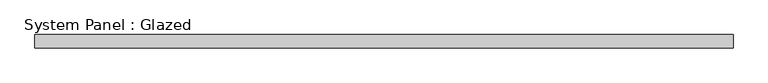
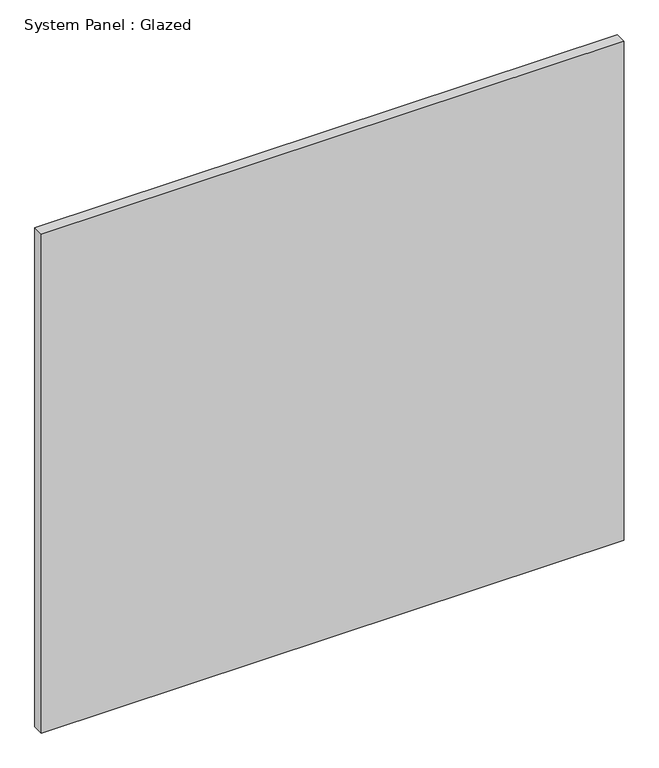
"""IFC4 building model written with IfcOpenShell, lengths in millimetres: plate geometry, System Panel : Glazed."""

from ifc_helpers import new_model, si_unit, origin, origin_with_axes, place, context, project, spatial, polyline, outline, extrude, source, transform, mapped, element, save


def system_panel_glazed_61697952(model_context):
    return source(origin(), model_context, "Body", "SweptSolid", [
        extrude(outline(polyline([(673.8477062, 19.05), (-673.8477062, 19.05), (-673.8477062, 44.45), (673.8477062, 44.45), (673.8477062, 19.05)])), origin_with_axes(), (0.0, 0.0, 1.0), 1219.2),
    ])


if __name__ == "__main__":
    model = new_model("IFC4")
    model_context = context("Model", 3, world=origin())
    ifc_project = project(units=[si_unit("LENGTHUNIT", "METRE", prefix="MILLI")], contexts=[model_context])
    site = spatial("IfcSite", under=ifc_project)
    building = spatial("IfcBuilding", under=site)
    placement = place(None, origin())
    system_panel_glazed_shape = system_panel_glazed_61697952(model_context)
    element("IfcPlate", 1, ObjectType="System Panel : Glazed", at=placement, inside=building, context=model_context, shape_type="MappedRepresentation", body=[
        mapped(system_panel_glazed_shape, transform((0.0, 0.0, 0.0), x_axis=(1.0, 0.0, 0.0), y_axis=(0.0, 1.0, 0.0), z_axis=(0.0, 0.0, 1.0))),
    ])
    save(model, "model.ifc")

# Revit data of these elements
# Type "System Panel : Glazed"
#   Construction Type Id = "GSP4R"
#   Analytic Construction = "1/8 in Pilkington single glazing"
#   Visual Light Transmittance = 0.9
#   Solar Heat Gain Coefficient = 0.86
#   Heat Transfer Coefficient (U) = 1.18115 BTU/(h·ft²·°F)
# Element 1 (IfcPlate, "System Panel : Glazed")
#   Materials on its faces: "Glass"
# Materials
#   "Glass": class "Glass", colour RGB 0 128 192, transparency 0.75, Description = "Soda Lime Glass", Cost = 0
